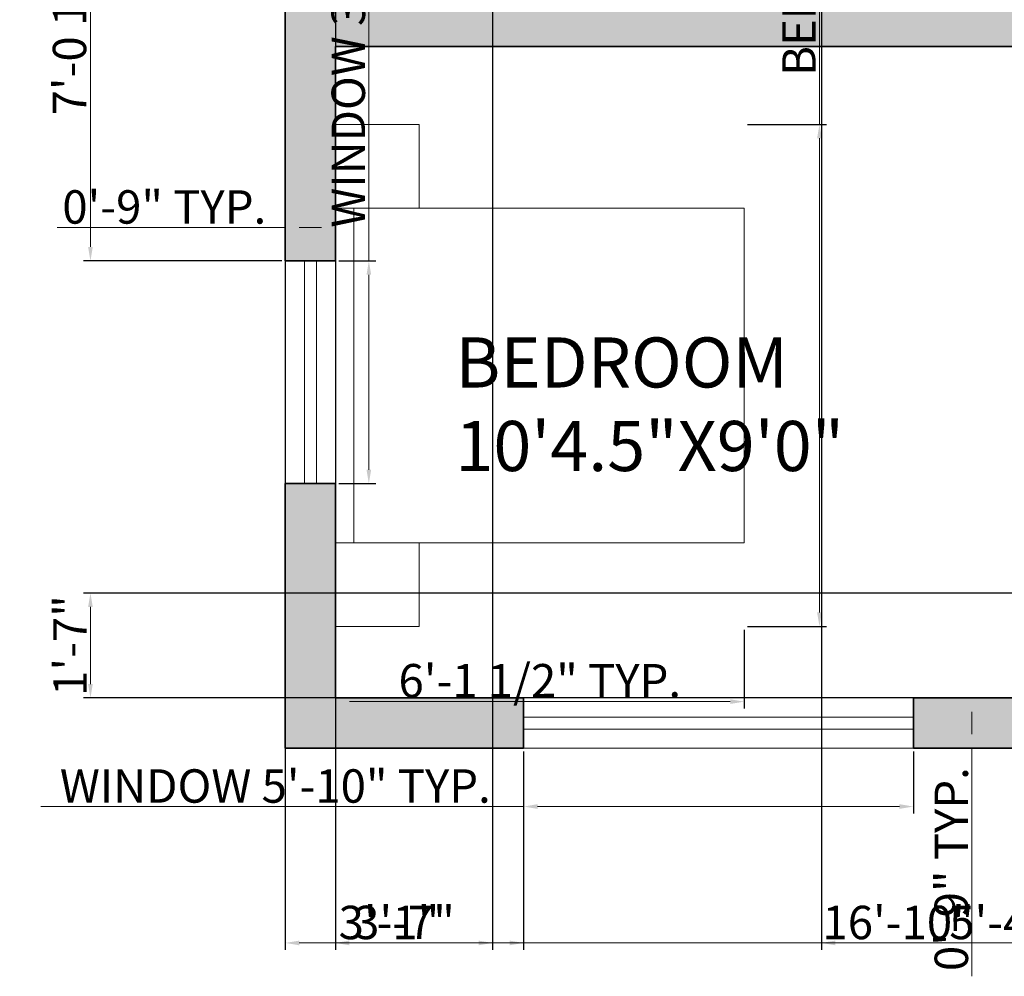
# Model space of a CAD drawing. Units: inches. Extents: x 2696 to 3240, y 1564 to 2310.
# Tile 1 of 76: x 2698 to 2875, y 1564 to 1736. Entities that reach past the tile are written whole.
import ezdxf

# ---------------------------------------------------------------- set-up
doc = ezdxf.new("R2010")
doc.units = ezdxf.units.IN
for name, color, linetype, lineweight in [('A-ANNO-DIMS', 3, 'Continuous', 18), ('A-AREA-IDEN', 7, 'Continuous', 18), ('A-FURN', 251, 'Continuous', 13), ('A-WALL', 7, 'Continuous', 35), ('A-WALL-PATT', 9, 'Continuous', 13), ('WINDOW', 2, 'Continuous', 18)]:
    doc.layers.add(name, color=color, linetype=linetype, lineweight=lineweight)
doc.styles.add('TIMES NEW', font='times.ttf')
doc.styles.add('YQ_DIM', font='SUPEROS.SHX', dxfattribs={"width": 0.8, "bigfont": 'HZDX.SHX'})
doc.dimstyles.new('Siddhuu', dxfattribs={"dimtxt": 6, "dimasz": 2.5, "dimexe": 1.25, "dimexo": 0.625, "dimtad": 1, "dimdec": 1, "dimlunit": 4, "dimtxsty": 'TIMES NEW', "dimcen": 2.5, "dimclrd": 256, "dimclre": 1, "dimclrt": 7, "dimadec": 0, "dimazin": 0, "dimtfac": 1, "dimtdec": 1, "dimtmove": 0, "dimatfit": 3, "dimfxl": 1, "dimtolj": 1, "dimlwd": -1, "dimarcsym": 0})

# ---------------------------------------------------------------- blocks, each defined once
blk = doc.blocks.new('WD_WIN4')
for p, q in [((-0.5, 0.5), (0.5, 0.5)), ((-0.5, 0.12), (0.5, 0.12)), ((-0.5, -0.12), (0.5, -0.12)), ((-0.5, -0.5), (0.5, -0.5))]:
    blk.add_line(p, q)
blk = doc.blocks.new('BED-DOUBLE-WITH-NIGHTSTANDS')
for points in [[(0, 75.13), (0, 90.16), (15.03, 90.16), (15.03, 75.13)], [(3.28, 15.03), (3.28, 75.13), (73.4, 75.13), (73.4, 15.03)], [(0, 15.03), (0, 0), (15.03, 0), (15.03, 15.03)]]:
    blk.add_lwpolyline(points, close=True)
blk = doc.blocks.new('*D22')
at = {"layer": 'A-ANNO-DIMS', "transparency": 16777216}
for p, q in [((2760.61, 1692.7), (2760.61, 1774.98)), ((2760.61, 1655.2), (2760.61, 1690.2))]:
    blk.add_line(p, q, dxfattribs=at)
at = {"layer": 'A-ANNO-DIMS', "color": 1, "lineweight": -2, "transparency": 16777216}
for p, q in [((2755.24, 1692.7), (2761.86, 1692.7)), ((2755.24, 1652.7), (2761.86, 1652.7))]:
    blk.add_line(p, q, dxfattribs=at)
at = {"layer": 'A-ANNO-DIMS', "transparency": 16777216}
for points in [[(2760.19, 1690.2), (2761.03, 1690.2), (2760.61, 1692.7)], [(2760.19, 1655.2), (2761.03, 1655.2), (2760.61, 1652.7)]]:
    blk.add_solid(points, dxfattribs=at)
at = {"layer": 'Defpoints', "color": 0, "transparency": 16777216}
for p in [(2754.61, 1692.7), (2760.61, 1692.7), (2754.61, 1652.7)]:
    blk.add_point(p, dxfattribs=at)
at = {"layer": 'A-ANNO-DIMS', "color": 7, "transparency": 16777216, "insert": (2756.92, 1735.09), "char_height": 6, "attachment_point": 5, "rotation": 90, "style": 'TIMES NEW'}
blk.add_mtext('\\A1;WINDOW 3\'-4" TYP.', dxfattribs=at)
blk = doc.blocks.new('*D23')
at = {"layer": 'A-ANNO-DIMS', "color": 1, "lineweight": -2, "transparency": 16777216}
for p, q in [((2745.61, 1693.33), (2745.61, 1699.95)), ((2754.61, 1693.33), (2754.61, 1699.95))]:
    blk.add_line(p, q, dxfattribs=at)
at = {"layer": 'A-ANNO-DIMS', "transparency": 16777216}
for p, q in [((2745.61, 1698.7), (2704.62, 1698.7)), ((2752.11, 1698.7), (2748.11, 1698.7))]:
    blk.add_line(p, q, dxfattribs=at)
for points in [[(2748.11, 1699.12), (2748.11, 1698.28), (2745.61, 1698.7)], [(2752.11, 1699.12), (2752.11, 1698.28), (2754.61, 1698.7)]]:
    blk.add_solid(points, dxfattribs=at)
at = {"layer": 'Defpoints', "color": 0, "transparency": 16777216}
for p in [(2745.61, 1698.7), (2745.61, 1692.7), (2754.61, 1692.7)]:
    blk.add_point(p, dxfattribs=at)
at = {"layer": 'A-ANNO-DIMS', "color": 7, "transparency": 16777216, "insert": (2723.87, 1702.39), "char_height": 6, "attachment_point": 5, "style": 'TIMES NEW'}
blk.add_mtext('\\A1;0\'-9" TYP.', dxfattribs=at)
blk = doc.blocks.new('*D24')
at = {"layer": 'A-ANNO-DIMS', "color": 1, "lineweight": -2, "transparency": 16777216}
for p, q in [((2788.41, 1604.58), (2788.41, 1593.45)), ((2858.41, 1604.58), (2858.41, 1593.45))]:
    blk.add_line(p, q, dxfattribs=at)
at = {"layer": 'A-ANNO-DIMS', "transparency": 16777216}
for p, q in [((2788.41, 1594.7), (2701.7, 1594.7)), ((2855.91, 1594.7), (2790.91, 1594.7))]:
    blk.add_line(p, q, dxfattribs=at)
for points in [[(2790.91, 1595.12), (2790.91, 1594.28), (2788.41, 1594.7)], [(2855.91, 1595.12), (2855.91, 1594.28), (2858.41, 1594.7)]]:
    blk.add_solid(points, dxfattribs=at)
at = {"layer": 'Defpoints', "color": 0, "transparency": 16777216}
for p in [(2788.41, 1605.2), (2858.41, 1605.2), (2788.41, 1594.7)]:
    blk.add_point(p, dxfattribs=at)
at = {"layer": 'A-ANNO-DIMS', "color": 7, "transparency": 16777216, "insert": (2743.81, 1598.39), "char_height": 6, "attachment_point": 5, "style": 'TIMES NEW'}
blk.add_mtext('\\A1;WINDOW 5\'-10" TYP.', dxfattribs=at)
blk = doc.blocks.new('*D25')
at = {"layer": 'A-ANNO-DIMS', "color": 1, "lineweight": -2, "transparency": 16777216}
for p, q in [((2859.04, 1614.2), (2870.16, 1614.2)), ((2859.04, 1605.2), (2870.16, 1605.2))]:
    blk.add_line(p, q, dxfattribs=at)
at = {"layer": 'A-ANNO-DIMS', "transparency": 16777216}
for p, q in [((2868.91, 1611.7), (2868.91, 1607.7)), ((2868.91, 1605.2), (2868.91, 1564.21))]:
    blk.add_line(p, q, dxfattribs=at)
for points in [[(2868.49, 1611.7), (2869.33, 1611.7), (2868.91, 1614.2)], [(2868.49, 1607.7), (2869.33, 1607.7), (2868.91, 1605.2)]]:
    blk.add_solid(points, dxfattribs=at)
at = {"layer": 'Defpoints', "color": 0, "transparency": 16777216}
for p in [(2858.41, 1614.2), (2858.41, 1605.2), (2868.91, 1605.2)]:
    blk.add_point(p, dxfattribs=at)
at = {"layer": 'A-ANNO-DIMS', "color": 7, "transparency": 16777216, "insert": (2865.22, 1583.46), "char_height": 6, "attachment_point": 5, "rotation": 90, "style": 'TIMES NEW'}
blk.add_mtext('\\A1;0\'-9" TYP.', dxfattribs=at)
blk = doc.blocks.new('*D46')
at = {"layer": 'A-ANNO-DIMS', "transparency": 16777216}
for p, q in [((2841.54, 1717.22), (2841.54, 1851.66)), ((2841.54, 1629.56), (2841.54, 1714.72))]:
    blk.add_line(p, q, dxfattribs=at)
at = {"layer": 'A-ANNO-DIMS', "color": 1, "lineweight": -2, "transparency": 16777216}
for p, q in [((2828.64, 1717.22), (2842.79, 1717.22)), ((2828.64, 1627.06), (2842.79, 1627.06))]:
    blk.add_line(p, q, dxfattribs=at)
at = {"layer": 'A-ANNO-DIMS', "transparency": 16777216}
for points in [[(2841.12, 1714.72), (2841.96, 1714.72), (2841.54, 1717.22)], [(2841.12, 1629.56), (2841.96, 1629.56), (2841.54, 1627.06)]]:
    blk.add_solid(points, dxfattribs=at)
at = {"layer": 'Defpoints', "color": 0, "transparency": 16777216}
for p in [(2828.01, 1717.22), (2841.54, 1717.22), (2828.01, 1627.06)]:
    blk.add_point(p, dxfattribs=at)
at = {"layer": 'A-ANNO-DIMS', "color": 7, "transparency": 16777216, "insert": (2837.85, 1785.69), "char_height": 6, "attachment_point": 5, "rotation": 90, "style": 'TIMES NEW'}
blk.add_mtext('\\A1;BED & NIGHTSTANDS 7\'-6" TYP.', dxfattribs=at)
blk = doc.blocks.new('*D47')
at = {"layer": 'A-ANNO-DIMS', "color": 1, "lineweight": -2, "transparency": 16777216}
for p, q in [((2754.61, 1626.44), (2754.61, 1612.29)), ((2828.01, 1626.44), (2828.01, 1612.29))]:
    blk.add_line(p, q, dxfattribs=at)
at = {"layer": 'A-ANNO-DIMS', "transparency": 16777216}
blk.add_line((2757.11, 1613.54), (2825.51, 1613.54), dxfattribs=at)
for points in [[(2757.11, 1613.96), (2757.11, 1613.12), (2754.61, 1613.54)], [(2825.51, 1613.96), (2825.51, 1613.12), (2828.01, 1613.54)]]:
    blk.add_solid(points, dxfattribs=at)
at = {"layer": 'Defpoints', "color": 0, "transparency": 16777216}
for p in [(2754.61, 1627.06), (2828.01, 1627.06), (2828.01, 1613.54)]:
    blk.add_point(p, dxfattribs=at)
at = {"layer": 'A-ANNO-DIMS', "color": 7, "transparency": 16777216, "insert": (2791.31, 1617.3), "char_height": 6, "attachment_point": 5, "style": 'TIMES NEW'}
blk.add_mtext('\\A1;6\'-1 1/2" TYP.', dxfattribs=at)
blk = doc.blocks.new('*D57')
at = {"layer": 'A-ANNO-DIMS', "color": 1, "lineweight": -2, "transparency": 16777216}
for p, q in [((2754.61, 2018.58), (2754.61, 1568.95)), ((2956.71, 2018.58), (2956.71, 1568.95))]:
    blk.add_line(p, q, dxfattribs=at)
at = {"layer": 'A-ANNO-DIMS', "transparency": 16777216}
blk.add_line((2757.11, 1570.2), (2954.21, 1570.2), dxfattribs=at)
for points in [[(2757.11, 1570.62), (2757.11, 1569.78), (2754.61, 1570.2)], [(2954.21, 1570.62), (2954.21, 1569.78), (2956.71, 1570.2)]]:
    blk.add_solid(points, dxfattribs=at)
at = {"layer": 'Defpoints', "color": 0, "transparency": 16777216}
for p in [(2754.61, 2019.2), (2956.71, 2019.2), (2956.71, 1570.2)]:
    blk.add_point(p, dxfattribs=at)
at = {"layer": 'A-ANNO-DIMS', "color": 7, "transparency": 16777216, "insert": (2855.66, 1573.88), "char_height": 6, "attachment_point": 5, "style": 'TIMES NEW'}
blk.add_mtext('\\A1;16\'-10"', dxfattribs=at)
blk = doc.blocks.new('*D68')
at = {"layer": 'A-ANNO-DIMS', "color": 1, "lineweight": -2, "transparency": 16777216}
for p, q in [((2745.61, 2261.58), (2745.61, 1568.95)), ((2782.83, 2261.58), (2782.83, 1568.95))]:
    blk.add_line(p, q, dxfattribs=at)
at = {"layer": 'A-ANNO-DIMS', "transparency": 16777216}
blk.add_line((2748.11, 1570.2), (2780.33, 1570.2), dxfattribs=at)
for points in [[(2748.11, 1570.62), (2748.11, 1569.78), (2745.61, 1570.2)], [(2780.33, 1570.62), (2780.33, 1569.78), (2782.83, 1570.2)]]:
    blk.add_solid(points, dxfattribs=at)
at = {"layer": 'Defpoints', "color": 0, "transparency": 16777216}
for p in [(2745.61, 2262.2), (2782.83, 2262.2), (2782.83, 1570.2)]:
    blk.add_point(p, dxfattribs=at)
at = {"layer": 'A-ANNO-DIMS', "color": 7, "transparency": 16777216, "insert": (2764.22, 1573.88), "char_height": 6, "attachment_point": 5, "style": 'TIMES NEW'}
blk.add_mtext('\\A1;3\'-1"', dxfattribs=at)
blk = doc.blocks.new('*D69')
at = {"layer": 'A-ANNO-DIMS', "color": 1, "lineweight": -2, "transparency": 16777216}
for p, q in [((2841.89, 2261.58), (2841.89, 1568.95)), ((2905.91, 2261.58), (2905.91, 1568.95))]:
    blk.add_line(p, q, dxfattribs=at)
at = {"layer": 'A-ANNO-DIMS', "transparency": 16777216}
blk.add_line((2844.39, 1570.2), (2903.41, 1570.2), dxfattribs=at)
for points in [[(2844.39, 1570.62), (2844.39, 1569.78), (2841.89, 1570.2)], [(2903.41, 1570.62), (2903.41, 1569.78), (2905.91, 1570.2)]]:
    blk.add_solid(points, dxfattribs=at)
at = {"layer": 'Defpoints', "color": 0, "transparency": 16777216}
for p in [(2841.89, 2262.2), (2905.91, 2262.2), (2905.91, 1570.2)]:
    blk.add_point(p, dxfattribs=at)
at = {"layer": 'A-ANNO-DIMS', "color": 7, "transparency": 16777216, "insert": (2873.9, 1573.88), "char_height": 6, "attachment_point": 5, "style": 'TIMES NEW'}
blk.add_mtext('\\A1;5\'-4"', dxfattribs=at)
blk = doc.blocks.new('*D74')
at = {"layer": 'A-ANNO-DIMS', "color": 1, "lineweight": -2, "transparency": 16777216}
for p, q in [((2744.99, 1777.2), (2709.36, 1777.2)), ((2744.99, 1692.7), (2709.36, 1692.7))]:
    blk.add_line(p, q, dxfattribs=at)
at = {"layer": 'A-ANNO-DIMS', "transparency": 16777216}
blk.add_line((2710.61, 1774.7), (2710.61, 1695.2), dxfattribs=at)
for points in [[(2710.19, 1774.7), (2711.03, 1774.7), (2710.61, 1777.2)], [(2710.19, 1695.2), (2711.03, 1695.2), (2710.61, 1692.7)]]:
    blk.add_solid(points, dxfattribs=at)
at = {"layer": 'Defpoints', "color": 0, "transparency": 16777216}
for p in [(2745.61, 1777.2), (2710.61, 1692.7), (2745.61, 1692.7)]:
    blk.add_point(p, dxfattribs=at)
at = {"layer": 'A-ANNO-DIMS', "color": 7, "transparency": 16777216, "insert": (2706.85, 1734.95), "char_height": 6, "attachment_point": 5, "rotation": 90, "style": 'TIMES NEW'}
blk.add_mtext('\\A1;7\'-0 1/2"', dxfattribs=at)
blk = doc.blocks.new('*D75')
at = {"layer": 'A-ANNO-DIMS', "color": 1, "lineweight": -2, "transparency": 16777216}
for p, q in [((2745.61, 1604.58), (2745.61, 1568.95)), ((2788.41, 1604.58), (2788.41, 1568.95))]:
    blk.add_line(p, q, dxfattribs=at)
at = {"layer": 'A-ANNO-DIMS', "transparency": 16777216}
blk.add_line((2748.11, 1570.2), (2785.91, 1570.2), dxfattribs=at)
for points in [[(2748.11, 1570.62), (2748.11, 1569.78), (2745.61, 1570.2)], [(2785.91, 1570.62), (2785.91, 1569.78), (2788.41, 1570.2)]]:
    blk.add_solid(points, dxfattribs=at)
at = {"layer": 'Defpoints', "color": 0, "transparency": 16777216}
for p in [(2745.61, 1605.2), (2788.41, 1605.2), (2788.41, 1570.2)]:
    blk.add_point(p, dxfattribs=at)
at = {"layer": 'A-ANNO-DIMS', "color": 7, "transparency": 16777216, "insert": (2767.01, 1573.89), "char_height": 6, "attachment_point": 5, "style": 'TIMES NEW'}
blk.add_mtext('\\A1;3\'-7"', dxfattribs=at)
blk = doc.blocks.new('*D81')
at = {"layer": 'A-ANNO-DIMS', "color": 1, "lineweight": -2, "transparency": 16777216}
for p, q in [((3189.99, 1633.05), (2709.36, 1633.05)), ((3189.99, 1614.2), (2709.36, 1614.2))]:
    blk.add_line(p, q, dxfattribs=at)
at = {"layer": 'A-ANNO-DIMS', "transparency": 16777216}
blk.add_line((2710.61, 1616.7), (2710.61, 1630.55), dxfattribs=at)
for points in [[(2710.19, 1630.55), (2711.03, 1630.55), (2710.61, 1633.05)], [(2710.19, 1616.7), (2711.03, 1616.7), (2710.61, 1614.2)]]:
    blk.add_solid(points, dxfattribs=at)
at = {"layer": 'Defpoints', "color": 0, "transparency": 16777216}
for p in [(2710.61, 1633.05), (3190.61, 1633.05), (3190.61, 1614.2)]:
    blk.add_point(p, dxfattribs=at)
at = {"layer": 'A-ANNO-DIMS', "color": 7, "transparency": 16777216, "insert": (2706.93, 1623.62), "char_height": 6, "attachment_point": 5, "rotation": 90, "style": 'TIMES NEW'}
blk.add_mtext('\\A1;1\'-7"', dxfattribs=at)

msp = doc.modelspace()

# ---------------------------------------------------------------- hatches: boundary and pattern name
at = {"layer": 'A-WALL-PATT', "transparency": 33554556}
h = msp.add_hatch(color=256, dxfattribs=at)
h.dxf.hatch_style = 1
h.paths.add_polyline_path([(2879.11, 2253.2), (2905.91, 2253.2), (2905.91, 2262.2), (2841.89, 2262.2), (2841.89, 2253.2), (2870.11, 2253.2), (2870.11, 2176.6), (2965.71, 2176.6), (2965.71, 2206.7), (2973.58, 2206.7), (2973.58, 2215.7), (2965.71, 2215.7), (2965.71, 2262.2), (2929.91, 2262.2), (2929.91, 2253.2), (2956.71, 2253.2), (2956.71, 2185.6), (2879.11, 2185.6)])
h.paths.add_polyline_path([(2782.83, 2262.2), (2745.61, 2262.2), (2745.61, 2228.73), (2754.61, 2228.73), (2754.61, 2253.2), (2782.83, 2253.2)])
h.paths.add_polyline_path([(2754.61, 2136.2), (2965.71, 2136.2), (2965.71, 2145.2), (2879.11, 2145.2), (2879.11, 2147.07), (2877.34, 2147.07), (2870.11, 2147.07), (2870.11, 2145.2), (2754.61, 2145.2), (2754.61, 2169.67), (2745.61, 2169.67), (2745.61, 2000.2), (2754.61, 2000.2), (2754.61, 2019.2), (2849.08, 2019.2), (2849.08, 2023.7), (2841.21, 2023.7), (2841.21, 2051.83), (2836.71, 2051.83), (2836.71, 2023.7), (2754.61, 2023.7), (2754.61, 2091.2), (2836.71, 2091.2), (2836.71, 2087.83), (2841.21, 2087.83), (2841.21, 2095.7), (2754.61, 2095.7)])
h.paths.add_polyline_path([(2965.71, 2136.2), (2956.71, 2136.2), (2956.71, 2023.7), (2885.08, 2023.7), (2885.08, 2019.2), (2956.71, 2019.2), (2956.71, 1950.58), (2965.71, 1950.58), (2965.71, 1980.2), (2973.58, 1980.2), (2973.58, 1989.2), (2965.71, 1989.2)])
h.paths.add_polyline_path([(2754.61, 1906.7), (2880.21, 1906.7), (2884.71, 1906.7), (2956.71, 1906.7), (2956.71, 1792.7), (2944.71, 1792.7), (2944.71, 1783.7), (2956.71, 1783.7), (2956.71, 1740.2), (2884.71, 1740.2), (2884.71, 1783.7), (2896.71, 1783.7), (2896.71, 1792.7), (2884.71, 1792.7), (2884.71, 1846.7), (2880.21, 1846.7), (2880.21, 1740.2), (2754.61, 1740.2), (2754.61, 1777.2), (2745.61, 1777.2), (2745.61, 1692.7), (2754.61, 1692.7), (2754.61, 1731.2), (2956.71, 1731.2), (2956.71, 1723.33), (2965.71, 1723.33), (2965.71, 1884.2), (2973.58, 1884.2), (2973.58, 1893.2), (2965.71, 1893.2), (2965.71, 1914.58), (2956.71, 1914.58), (2956.71, 1911.2), (2754.61, 1911.2), (2754.61, 1930.2), (2745.61, 1930.2), (2745.61, 1817.2), (2754.61, 1817.2), (2754.61, 1854.2), (2826.61, 1854.2), (2826.61, 1868.83), (2822.11, 1868.83), (2822.11, 1858.7), (2754.61, 1858.7)])
h.paths.add_polyline_path([(2965.71, 1656.2), (3008.24, 1656.2), (3008.24, 1665.2), (2965.71, 1665.2), (2965.71, 1693.33), (2956.71, 1693.33), (2956.71, 1686.2), (2934.58, 1686.2), (2934.58, 1681.7), (2956.71, 1681.7), (2956.71, 1614.2), (2896.71, 1614.2), (2896.71, 1681.7), (2904.58, 1681.7), (2904.58, 1686.2), (2892.21, 1686.2), (2892.21, 1614.2), (2858.41, 1614.2), (2858.41, 1605.2), (2965.71, 1605.2)])
h.paths.add_polyline_path([(2788.41, 1614.2), (2754.61, 1614.2), (2754.61, 1652.7), (2745.61, 1652.7), (2745.61, 1605.2), (2788.41, 1605.2)])
h.paths.add_polyline_path([(3199.61, 1633.05), (3190.61, 1633.05), (3190.61, 1614.2), (3082.61, 1614.2), (3082.61, 1665.2), (3070.24, 1665.2), (3070.24, 1656.2), (3078.11, 1656.2), (3078.11, 1605.2), (3199.61, 1605.2)])
h.paths.add_polyline_path([(3199.61, 1702.05), (3190.61, 1702.05), (3190.61, 1699.7), (3106.61, 1699.7), (3106.61, 1747.7), (3190.61, 1747.7), (3190.61, 1752.2), (3082.61, 1752.2), (3082.61, 1760.08), (3078.11, 1760.08), (3078.11, 1747.7), (3102.11, 1747.7), (3102.11, 1699.7), (3078.11, 1699.7), (3078.11, 1695.2), (3190.61, 1695.2), (3190.61, 1676.35), (3199.61, 1676.35)])
h.paths.add_polyline_path([(3199.61, 1783.2), (3190.61, 1783.2), (3190.61, 1745.35), (3199.61, 1745.35)])
h.paths.add_polyline_path([(3082.61, 1884.2), (3190.61, 1884.2), (3190.61, 1853.2), (3199.61, 1853.2), (3199.61, 1901.7), (3190.61, 1901.7), (3190.61, 1893.2), (3005.58, 1893.2), (3005.58, 1891.28), (3005.58, 1884.2), (3078.11, 1884.2), (3078.11, 1792.08), (3082.61, 1792.08)])
h.paths.add_polyline_path([(3199.61, 1994.7), (3190.61, 1994.7), (3190.61, 1989.2), (3073.71, 1989.2), (3073.71, 2034.2), (3069.21, 2034.2), (3069.21, 1989.2), (3005.58, 1989.2), (3005.58, 1980.2), (3190.61, 1980.2), (3190.61, 1971.7), (3199.61, 1971.7)])
h.paths.add_polyline_path([(3199.61, 2155.2), (3190.61, 2155.2), (3190.61, 2064.7), (3199.61, 2064.7)])
h.paths.add_polyline_path([(3190.61, 2074.7), (3106.61, 2074.7), (3106.61, 2122.7), (3190.61, 2122.7), (3190.61, 2127.2), (3082.71, 2127.2), (3082.71, 2135.08), (3073.71, 2135.08), (3073.71, 2122.7), (3102.11, 2122.7), (3102.11, 2074.7), (3069.21, 2074.7), (3069.21, 2070.2), (3190.61, 2070.2)])
h.paths.add_polyline_path([(3082.71, 2253.2), (3190.61, 2253.2), (3190.61, 2225.2), (3199.61, 2225.2), (3199.61, 2262.2), (3073.71, 2262.2), (3073.71, 2215.7), (3035.58, 2215.7), (3035.58, 2206.7), (3073.71, 2206.7), (3073.71, 2171.08), (3082.71, 2171.08)])

# ---------------------------------------------------------------- linework, layer by layer
at = {"layer": 'A-WALL'}
for p, q in [((2745.61, 1692.7), (2745.61, 1777.2)), ((2754.61, 1731.2), (2956.71, 1731.2)), ((2754.61, 1692.7), (2754.61, 1731.2)), ((2754.61, 1692.7), (2745.61, 1692.7)), ((2745.61, 1605.2), (2745.61, 1652.7)), ((2754.61, 1652.7), (2745.61, 1652.7)), ((2754.61, 1614.2), (2754.61, 1652.7)), ((2754.61, 1614.2), (2788.41, 1614.2)), ((2788.41, 1614.2), (2788.41, 1605.2)), ((2858.41, 1614.2), (2892.21, 1614.2)), ((2858.41, 1614.2), (2858.41, 1605.2)), ((2745.61, 1605.2), (2788.41, 1605.2)), ((2858.41, 1605.2), (2965.71, 1605.2))]:
    msp.add_line(p, q, dxfattribs=at)

# ---------------------------------------------------------------- block references
at = {"layer": 'A-FURN'}
msp.add_blockref('BED-DOUBLE-WITH-NIGHTSTANDS', (2754.61, 1627.06), dxfattribs=at)
at = {"layer": 'WINDOW', "yscale": 9}
for p, xscale, zscale, rotation in [((2750.11, 1672.7), 40, 40, 90), ((2823.41, 1609.7), 70, 70, 180)]:
    msp.add_blockref('WD_WIN4', p, dxfattribs=dict(at, xscale=xscale, zscale=zscale, rotation=rotation))

# ---------------------------------------------------------------- texts
at = {"layer": 'A-AREA-IDEN', "insert": (2776.16, 1678.96), "char_height": 9, "attachment_point": 1, "style": 'YQ_DIM'}
msp.add_mtext_dynamic_manual_height_columns('BEDROOM\\P10\'4.5"X9\'0"', width=48.0032, gutter_width=12.5, heights=[0], dxfattribs=at)

# ---------------------------------------------------------------- dimensions: what is measured, and where the dimension line sits
at = {"layer": 'A-ANNO-DIMS'}
for base, p1, p2, picture, middle in [((2782.83, 1570.2), (2745.61, 2262.2), (2782.83, 2262.2), '*D68', (2764.22, 1573.88)), ((2905.91, 1570.2), (2841.89, 2262.2), (2905.91, 2262.2), '*D69', (2873.9, 1573.88)), ((2956.71, 1570.2), (2754.61, 2019.2), (2956.71, 2019.2), '*D57', (2855.66, 1573.88)), ((2788.41, 1570.2), (2745.61, 1605.2), (2788.41, 1605.2), '*D75', (2767.01, 1573.89))]:
    dim = msp.add_linear_dim(base=base, p1=p1, p2=p2, dimstyle='Siddhuu', override={"dimdec": 1, "dimlfac": 1, "dimrnd": 0, "dimzin": 1, "dimdsep": 46, "dimlunit": 4, "dimfrac": 2}, dxfattribs=at)
    dim.commit()
    dim.dimension.update_dxf_attribs({"geometry": picture, "text_midpoint": middle})
for base, p1, p2, angle, text, picture, middle in [((2841.54, 1717.22), (2828.01, 1627.06), (2828.01, 1717.22), 90, 'BED & NIGHTSTANDS <> TYP.', '*D46', (2837.85, 1785.69)), ((2760.61, 1692.7), (2754.61, 1652.7), (2754.61, 1692.7), 90, 'WINDOW <> TYP.', '*D22', (2756.92, 1735.09)), ((2745.61, 1698.7), (2754.61, 1692.7), (2745.61, 1692.7), 180, '<> TYP.', '*D23', (2723.87, 1702.39)), ((2868.91, 1605.2), (2858.41, 1614.2), (2858.41, 1605.2), 270, '<> TYP.', '*D25', (2865.22, 1583.46)), ((2788.41, 1594.7), (2858.41, 1605.2), (2788.41, 1605.2), 180, 'WINDOW <> TYP.', '*D24', (2743.81, 1598.39))]:
    dim = msp.add_linear_dim(base=base, p1=p1, p2=p2, angle=angle, text=text, dimstyle='Siddhuu', override={"dimdec": 1, "dimlfac": 1, "dimrnd": 0, "dimzin": 1, "dimdsep": 46, "dimlunit": 4, "dimfrac": 2}, dxfattribs=at)
    dim.commit()
    dim.dimension.update_dxf_attribs({"geometry": picture, "text_midpoint": middle})
for base, p1, p2, picture, middle in [((2710.61, 1692.7), (2745.61, 1777.2), (2745.61, 1692.7), '*D74', (2706.85, 1734.95)), ((2710.6114, 1633.0476), (3190.6114, 1614.2011), (3190.6114, 1633.0476), '*D81', (2706.9258, 1623.6243))]:
    dim = msp.add_linear_dim(base=base, p1=p1, p2=p2, angle=90, dimstyle='Siddhuu', override={"dimdec": 1, "dimlfac": 1, "dimrnd": 0, "dimzin": 1, "dimdsep": 46, "dimlunit": 4, "dimfrac": 2}, dxfattribs=at)
    dim.commit()
    dim.dimension.update_dxf_attribs({"geometry": picture, "text_midpoint": middle})
dim = msp.add_linear_dim(base=(2828.01, 1613.54), p1=(2754.61, 1627.06), p2=(2828.01, 1627.06), text='<> TYP.', dimstyle='Siddhuu', override={"dimdec": 1, "dimlfac": 1, "dimrnd": 0, "dimzin": 1, "dimdsep": 46, "dimlunit": 4, "dimfrac": 2}, dxfattribs=at)
dim.commit()
dim.dimension.update_dxf_attribs({"geometry": '*D47', "text_midpoint": (2791.31, 1617.3)})

doc.saveas('drawing.dxf')
